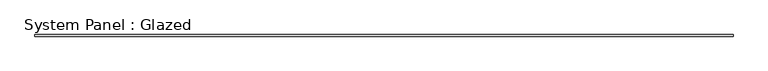
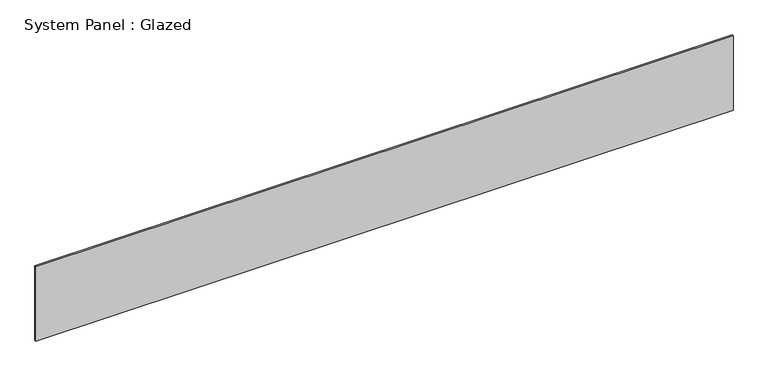
"""IFC4 building model written with IfcOpenShell, lengths in millimetres: plate geometry, System Panel : Glazed."""

from ifc_helpers import new_model, si_unit, origin, origin_with_axes, place, context, project, spatial, polyline, outline, extrude, source, transform, mapped, element, save


def system_panel_glazed_6c4e9d17(model_context):
    return source(origin(), model_context, "Body", "SweptSolid", [
        extrude(outline(polyline([(5410.2, 19.05), (-5410.2, 19.05), (-5410.2, 44.45), (5410.2, 44.45), (5410.2, 19.05)])), origin_with_axes(), (0.0, 0.0, 1.0), 1219.2),
    ])


if __name__ == "__main__":
    model = new_model("IFC4")
    model_context = context("Model", 3, world=origin())
    ifc_project = project(units=[si_unit("LENGTHUNIT", "METRE", prefix="MILLI")], contexts=[model_context])
    site = spatial("IfcSite", under=ifc_project)
    building = spatial("IfcBuilding", under=site)
    placement = place(None, origin())
    system_panel_glazed_shape = system_panel_glazed_6c4e9d17(model_context)
    element("IfcPlate", 1, ObjectType="System Panel : Glazed", at=placement, inside=building, context=model_context, shape_type="MappedRepresentation", body=[
        mapped(system_panel_glazed_shape, transform((0.0, 0.0, 0.0), x_axis=(1.0, 0.0, 0.0), y_axis=(0.0, 1.0, 0.0), z_axis=(0.0, 0.0, 1.0))),
    ])
    save(model, "model.ifc")

# Revit data of these elements
# Type "System Panel : Glazed"
#   Construction Type Id = "GSP4R"
#   Analytic Construction = "1/8 in Pilkington single glazing"
#   Visual Light Transmittance = 0.9
#   Solar Heat Gain Coefficient = 0.86
#   Heat Transfer Coefficient (U) = 1.18115 BTU/(h·ft²·°F)
# Element 1 (IfcPlate, "System Panel : Glazed")
#   Materials on its faces: "Glass"
# Materials
#   "Glass": class "Glass", colour RGB 0 128 192, transparency 0.75, Description = "Soda Lime Glass", Cost = 0
